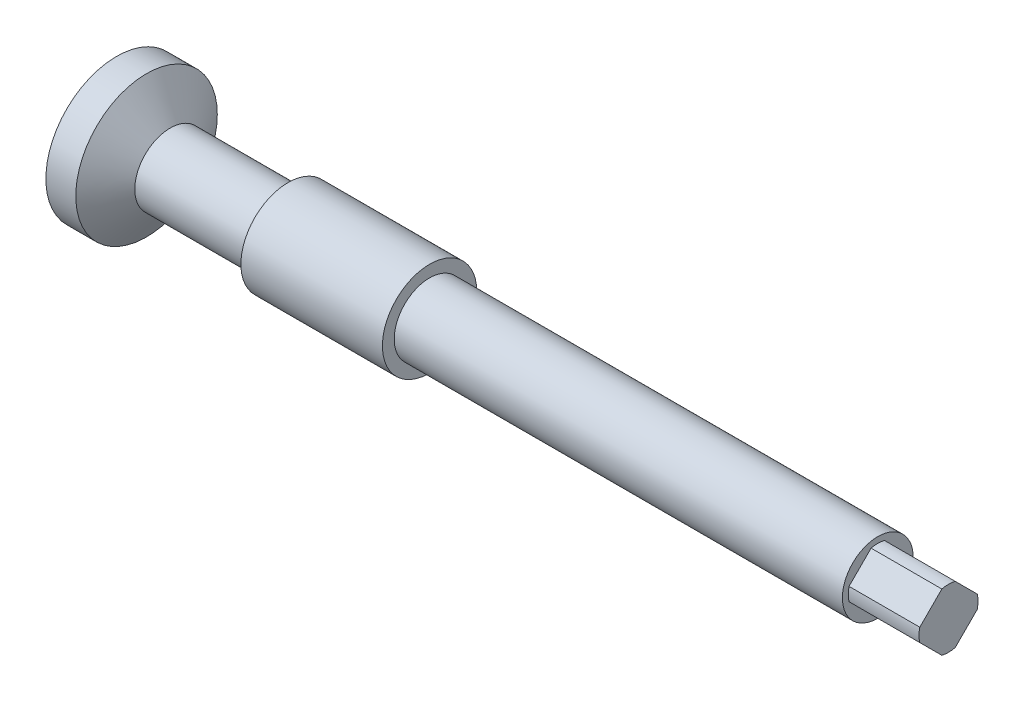
SolidWorks part; units mm, degrees
material "Plain Carbon Steel"
ref_plane "Front Plane" through (0, 0, 0) normal (0, 0, 1) x (1, 0, 0)
ref_plane "Top Plane" through (0, 0, 0) normal (0, 1, 0) x (1, 0, 0)
ref_plane "Right Plane" through (0, 0, 0) normal (1, 0, 0) x (0, 0, -1)
sketch "Spindle Profile Sketch" plane through (0, 0, 0) normal (0, 0, 1) x (1, 0, 0)
  line L0 (0, 0) -> (0, 2.5)
  line L1 (0, 2.5) -> (-6, 2.5)
  line L2 (-6, 2.5) -> (-6, 3)
  line L3 (-6, 3) -> (-44, 3)
  line L4 (-44, 3) -> (-44, 4)
  line L5 (-44, 4) -> (-56, 4)
  line L6 (-56, 4) -> (-56, 3)
  line L7 (-56, 3) -> (-66, 3)
  line L8 (-66, 3) -> (-68, 6)
  line L9 (-68, 6) -> (-70.5359, 6)
  line L12 (0, 0) -> (-74, 0) construction
  line L13 (-70.5359, 6) -> (-74, 0)
  line L14 (0, 0) -> (-74, 0)
  dimension "D1" = 74
  dimension "D2" = 6
  dimension "D3" = 38
  dimension "D4" = 12
  dimension "D5" = 10
  dimension "D6" = 2
  dimension "D7" = 5
  dimension "D8" = 6
  dimension "D9" = 8
  dimension "D10" = 6
  dimension "D11" = 12
  dimension "D12" = 60
revolve "Spindle Body Revolve" add sketch "Spindle Profile Sketch" angle 360 about L12
cosmetic thread "Cosmetic Thread1" parameters "D2"=6.619
sketch "Square Drive Sketch" plane through (0, 0, 0) normal (1, 0, 0) x (0, 0, -1)
  line L0 (-0.5, 2.5) -> (-2.5, 0.5)
  line L9 (0.5, -2.5) -> (-0.5, -2.5)
  line L10 (2.5, -0.5) -> (2.5, 0.5)
  line L11 (0.5, 2.5) -> (-0.5, 2.5)
  line L12 (-2.5, -0.5) -> (-2.5, 0.5)
  line L13 (2.5, -2.5) -> (-2.5, 2.5) construction
  line L14 (2.5, 2.5) -> (-2.5, -2.5) construction
  line L15 (2.5, 0.5) -> (0.5, 2.5)
  line L16 (2.5, -0.5) -> (0.5, -2.5)
  line L17 (-0.5, -2.5) -> (-2.5, -0.5)
  point P0 (0, 0)
  dimension "D1" = 5
  dimension "D2" = 5
extrude "Square Drive 5x5 Cut" cut sketch "Square Drive Sketch" against normal blind 6 flip side to cut
